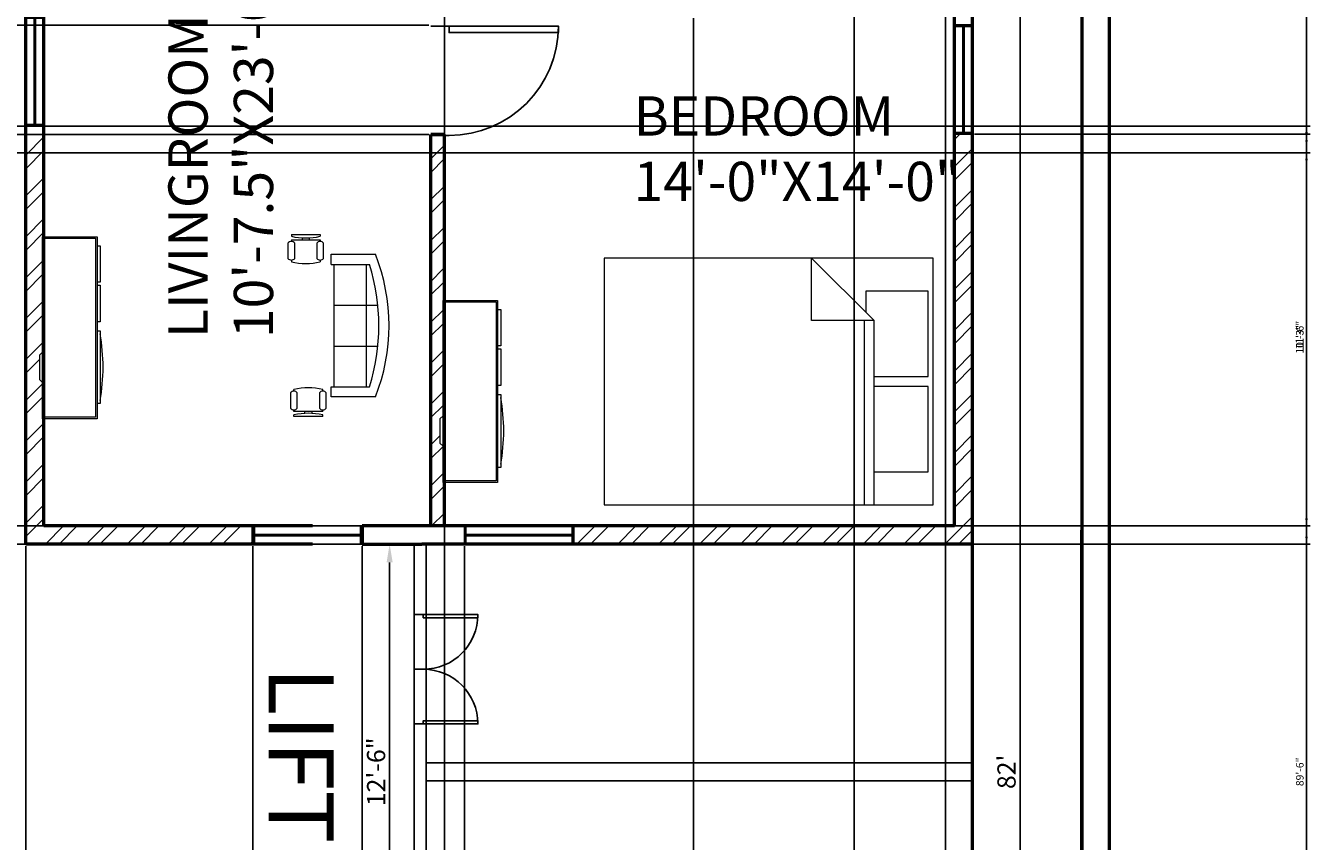
# Model space of a CAD drawing. Units: inches. Extents: x -12550 to 6516, y 1273 to 18700.
# Tile 6 of 19: x 2426 to 2849, y 1958 to 2227. Entities that reach past the tile are written whole.
import ezdxf

# ---------------------------------------------------------------- set-up
doc = ezdxf.new("R2010")
doc.units = ezdxf.units.IN
for name, color, linetype, lineweight in [('A-ANNO-DIMS', 2, 'Continuous', 18), ('A-AREA-IDEN', 1, 'Continuous', 18), ('A-DOOR', 5, 'Continuous', 25), ('A-EQPM', 4, 'Continuous', 25), ('A-FURN', 8, 'Continuous', 18), ('A-GLAZ', 3, 'Continuous', 25), ('A-WALL', 7, 'Continuous', 50), ('A-WALL-PATT', 8, 'Continuous', 13)]:
    doc.layers.add(name, color=color, linetype=linetype, lineweight=lineweight)
doc.styles.get("Standard").update_dxf_attribs({"font": 'arial.ttf'})
doc.dimstyles.new('ISO-25', dxfattribs={"dimtxt": 2.5, "dimasz": 2.5, "dimexe": 1.25, "dimexo": 0.625, "dimtad": 1, "dimlunit": 4, "dimtxsty": 'Standard', "dimcen": 2.5, "dimadec": 0, "dimazin": 0, "dimtfac": 1, "dimtmove": 0, "dimatfit": 3, "dimfxl": 1, "dimarcsym": 0})
pattern_1 = [(45, (-2e-13, 567), (-6.735192, 6.735192), []), (45, (4.49, 567), (-6.735192, 6.735192), [])]

# ---------------------------------------------------------------- blocks, each defined once
blk = doc.blocks.new('*U2')
for p, q in [((0, 0), (0, -5)), ((30, 0), (30, -5))]:
    blk.add_line(p, q)
blk.add_lwpolyline([(0, 0), (0, 30), (1.75, 30), (1.75, 0)], close=True)
blk.add_arc((0, 0), 30, 0, 90)
blk = doc.blocks.new('Bed - Queen')
for p, q in [((0, -80.00003), (0, 0)), ((0, 0), (59.99999, 0)), ((59.99999, 0), (59.99999, -80.00003)), ((7.99999, -1.2), (28.79998, -1.2)), ((7.99999, -14.4), (7.99999, -1.2)), ((28.79998, -1.2), (28.79998, -14.4)), ((31.19999, -1.2), (51.99999, -1.2)), ((31.19999, -14.4), (31.19999, -1.2)), ((51.99999, -1.2), (51.99999, -16.4)), ((0, -14.4), (44.8, -14.4)), ((59.99999, -29.6), (44.8, -14.4)), ((44.8, -14.4), (44.8, -29.6)), ((44.8, -16.8), (0, -16.8)), ((51.99999, -16.4), (46.79936, -16.4)), ((44.8, -29.6), (59.99999, -29.6)), ((59.99999, -80.00003), (0, -80.00003))]:
    blk.add_line(p, q)
blk = doc.blocks.new('Entertainment Center')
for p, q in [((-4, 0), (-5, -1)), ((4, 0), (-4, 0)), ((5, -1), (4, 0)), ((-17, -19), (-17, -1)), ((-17, -1), (43, -1)), ((-16.5, -18.5), (-16.5, -1.5)), ((-16.5, -1.5), (42.5, -1.5)), ((42.5, -1.5), (42.5, -18.5)), ((43, -1), (43, -19)), ((43, -19), (-17, -19)), ((42.5, -18.5), (-16.5, -18.5)), ((-12, -20), (-12, -19)), ((12, -20), (-12, -20)), ((12, -19), (12, -20)), ((15, -20), (15, -19)), ((27, -20), (15, -20)), ((27, -19), (27, -20)), ((28, -20), (28, -19)), ((40, -20), (28, -20)), ((40, -19), (40, -20))]:
    blk.add_line(p, q)
blk.add_arc((0, 40), 61, 259.6111, 280.3889)
blk = doc.blocks.new('Sofa - Roundback 7 ft.')
for p, q in [((-12.00002, -32.4421), (-12.00003, -6.5971)), ((11.99997, -32.4421), (11.99998, -6.5971)), ((-36.000027, -34), (-36.000027, -11.4696)), ((-35.999844, -13.3819), (35.9998, -13.3819)), ((35.99998, -34), (35.99998, -11.4696)), ((-36.000027, -32.4421), (35.99998, -32.4421))]:
    blk.add_line(p, q)
for points in [[(-36.000027, -34), (-42.000027, -34), (-42.000027, -8)], [(41.99998, -8), (41.99998, -34), (35.99998, -34)]]:
    blk.add_lwpolyline(points)
for centre, radius, start, end in [((0, -114.25), 114.25, 68.43141, 111.5686), ((-0.00001, -127.1968), 121.1968, 72.72033, 107.2797)]:
    blk.add_arc(centre, radius, start, end)
blk = doc.blocks.new('Chair - Desk')
for p, q in [((-8.5, 0), (-8.5, -1)), ((-8.5, 0), (8.5, 0)), ((8.5, 0), (8.5, -1)), ((-10.5, -5), (-10.5, -14)), ((-8.5, -3), (-8.5, -4)), ((-8.5, -3), (8.5, -3)), ((-6.5, -14), (-6.5, -5)), ((-2, -3), (-2, -1.9355)), ((2, -1.9576), (2, -3)), ((6.5, -5), (6.5, -14)), ((8.5, -3), (8.5, -4)), ((10.5, -14), (10.5, -5)), ((-8.5, -15), (-8.5, -16)), ((8.5, -15), (8.5, -16))]:
    blk.add_line(p, q)
for centre, radius, start, end in [((-8.5, -6.5), 2.5, 36.8699, 143.1301), ((0, 34.625), 36.625, 256.5803, 283.4197), ((8.5, -6.5), 2.5, 36.8699, 143.1301), ((-8.5, -12.5), 2.5, 216.8699, 323.1301), ((8.5, -12.5), 2.5, 216.8699, 323.1301), ((0, 19.625), 36.625, 256.5803, 283.4197)]:
    blk.add_arc(centre, radius, start, end)
blk = doc.blocks.new('*D14')
at = {"layer": 'A-ANNO-DIMS', "color": 0, "lineweight": -2, "transparency": 16777216}
for p, q in [((2553.06, 2056.25), (2544.35, 2056.25)), ((2545.6, 2050.25), (2545.6, 1912.25)), ((2553.06, 1906.25), (2544.35, 1906.25))]:
    blk.add_line(p, q, dxfattribs=at)
at = {"layer": 'A-ANNO-DIMS', "color": 0, "transparency": 16777216}
for points in [[(2544.6, 2050.25), (2546.6, 2050.25), (2545.6, 2056.25)], [(2544.6, 1912.25), (2546.6, 1912.25), (2545.6, 1906.25)]]:
    blk.add_solid(points, dxfattribs=at)
at = {"layer": 'Defpoints', "color": 0, "transparency": 16777216}
for p in [(2553.69, 2056.25), (2545.6, 1906.25), (2553.69, 1906.25)]:
    blk.add_point(p, dxfattribs=at)
at = {"layer": 'A-ANNO-DIMS', "color": 0, "transparency": 16777216, "insert": (2541.91, 1981.25), "char_height": 6, "attachment_point": 5, "rotation": 90}
blk.add_mtext('12\'-6"', dxfattribs=at)
blk = doc.blocks.new('*D16')
at = {"layer": 'A-ANNO-DIMS', "color": 0, "lineweight": -2, "transparency": 16777216}
for p, q in [((2738.31, 2473.25), (2754.56, 2473.25)), ((2753.31, 2467.25), (2753.31, 1495.25)), ((2738.31, 1489.25), (2754.56, 1489.25))]:
    blk.add_line(p, q, dxfattribs=at)
at = {"layer": 'A-ANNO-DIMS', "color": 0, "transparency": 16777216}
for points in [[(2752.31, 2467.25), (2754.31, 2467.25), (2753.31, 2473.25)], [(2752.31, 1495.25), (2754.31, 1495.25), (2753.31, 1489.25)]]:
    blk.add_solid(points, dxfattribs=at)
at = {"layer": 'Defpoints', "color": 0, "transparency": 16777216}
for p in [(2737.69, 2473.25), (2737.69, 1489.25), (2753.31, 1489.25)]:
    blk.add_point(p, dxfattribs=at)
at = {"layer": 'A-ANNO-DIMS', "color": 0, "transparency": 16777216, "insert": (2749.62, 1981.25), "char_height": 6, "attachment_point": 5, "rotation": 90}
blk.add_mtext("82'", dxfattribs=at)
blk = doc.blocks.new('WIN-3FT')
for p, q in [((0, 0), (0, 6)), ((0, 6), (36.02, 6)), ((0.5, 0), (0.5, 6)), ((35.52, 6), (35.52, 0)), ((36.02, 6), (36.02, 0)), ((36.02, 0), (0, 0)), ((35.52, 3.2), (0.5, 3.2)), ((35.52, 2.8), (0.5, 2.8))]:
    blk.add_line(p, q)
blk = doc.blocks.new('*D95')
at = {"layer": 'A-ANNO-DIMS', "color": 0, "lineweight": -2, "transparency": 16777216}
for p, q in [((2783.31, 2518.25), (2848.94, 2518.25)), ((2847.69, 1446.75), (2847.69, 2515.75)), ((2783.31, 1444.25), (2848.94, 1444.25))]:
    blk.add_line(p, q, dxfattribs=at)
at = {"layer": 'A-ANNO-DIMS', "color": 0, "transparency": 16777216}
for points in [[(2847.27, 2515.75), (2848.11, 2515.75), (2847.69, 2518.25)], [(2847.27, 1446.75), (2848.11, 1446.75), (2847.69, 1444.25)]]:
    blk.add_solid(points, dxfattribs=at)
at = {"layer": 'Defpoints', "color": 0, "transparency": 16777216}
for p in [(2782.69, 2518.25), (2847.69, 2518.25), (2782.69, 1444.25)]:
    blk.add_point(p, dxfattribs=at)
at = {"layer": 'A-ANNO-DIMS', "color": 0, "transparency": 16777216, "insert": (2845.79, 1981.25), "char_height": 2.5, "attachment_point": 5, "rotation": 90}
blk.add_mtext('89\'-6"', dxfattribs=at)
blk = doc.blocks.new('*D138')
at = {"layer": 'A-ANNO-DIMS', "color": 0, "lineweight": -2, "transparency": 16777216}
for p, q in [((2196.81, 2185.25), (2848.94, 2185.25)), ((2847.69, 2064.75), (2847.69, 2182.75)), ((2196.81, 2062.25), (2848.94, 2062.25))]:
    blk.add_line(p, q, dxfattribs=at)
at = {"layer": 'A-ANNO-DIMS', "color": 0, "transparency": 16777216}
for points in [[(2847.27, 2182.75), (2848.11, 2182.75), (2847.69, 2185.25)], [(2847.27, 2064.75), (2848.11, 2064.75), (2847.69, 2062.25)]]:
    blk.add_solid(points, dxfattribs=at)
at = {"layer": 'Defpoints', "color": 0, "transparency": 16777216}
for p in [(2196.19, 2185.25), (2847.69, 2185.25), (2196.19, 2062.25)]:
    blk.add_point(p, dxfattribs=at)
at = {"layer": 'A-ANNO-DIMS', "color": 0, "transparency": 16777216, "insert": (2845.79, 2123.75), "char_height": 2.5, "attachment_point": 5, "rotation": 90}
blk.add_mtext('10\'-3"', dxfattribs=at)
blk = doc.blocks.new('*D145')
at = {"layer": 'A-ANNO-DIMS', "color": 0, "lineweight": -2, "transparency": 16777216}
for p, q in [((2330.31, 2194.03), (2848.94, 2194.03)), ((2847.69, 2058.75), (2847.69, 2191.53)), ((2330.31, 2056.25), (2848.94, 2056.25))]:
    blk.add_line(p, q, dxfattribs=at)
at = {"layer": 'A-ANNO-DIMS', "color": 0, "transparency": 16777216}
for points in [[(2847.27, 2191.53), (2848.11, 2191.53), (2847.69, 2194.03)], [(2847.27, 2058.75), (2848.11, 2058.75), (2847.69, 2056.25)]]:
    blk.add_solid(points, dxfattribs=at)
at = {"layer": 'Defpoints', "color": 0, "transparency": 16777216}
for p in [(2329.69, 2194.03), (2847.69, 2194.03), (2329.69, 2056.25)]:
    blk.add_point(p, dxfattribs=at)
at = {"layer": 'A-ANNO-DIMS', "color": 0, "transparency": 16777216, "insert": (2845.79, 2125.14), "char_height": 2.5, "attachment_point": 5, "rotation": 90}
blk.add_mtext('11\'-6"', dxfattribs=at)
blk = doc.blocks.new('*D152')
at = {"layer": 'A-ANNO-DIMS', "color": 0, "lineweight": -2, "transparency": 16777216}
for p, q in [((2425.69, 2055.62), (2425.69, 1378)), ((2500.53, 2055.62), (2500.53, 1378)), ((2428.19, 1379.25), (2498.03, 1379.25))]:
    blk.add_line(p, q, dxfattribs=at)
at = {"layer": 'A-ANNO-DIMS', "color": 0, "transparency": 16777216}
for points in [[(2428.19, 1379.66), (2428.19, 1378.83), (2425.69, 1379.25)], [(2498.03, 1379.66), (2498.03, 1378.83), (2500.53, 1379.25)]]:
    blk.add_solid(points, dxfattribs=at)
at = {"layer": 'Defpoints', "color": 0, "transparency": 16777216}
for p in [(2425.69, 2056.25), (2500.53, 2056.25), (2500.53, 1379.25)]:
    blk.add_point(p, dxfattribs=at)
at = {"layer": 'A-ANNO-DIMS', "color": 0, "transparency": 16777216, "insert": (2463.11, 1381.15), "char_height": 2.5, "attachment_point": 5}
blk.add_mtext('6\'-3"', dxfattribs=at)
blk = doc.blocks.new('*D153')
at = {"layer": 'A-ANNO-DIMS', "color": 0, "lineweight": -2, "transparency": 16777216}
for p, q in [((2536.54, 2055.62), (2536.54, 1378)), ((2570.26, 2055.62), (2570.26, 1378)), ((2539.04, 1379.25), (2567.76, 1379.25))]:
    blk.add_line(p, q, dxfattribs=at)
at = {"layer": 'A-ANNO-DIMS', "color": 0, "transparency": 16777216}
for points in [[(2539.04, 1379.66), (2539.04, 1378.83), (2536.54, 1379.25)], [(2567.76, 1379.66), (2567.76, 1378.83), (2570.26, 1379.25)]]:
    blk.add_solid(points, dxfattribs=at)
at = {"layer": 'Defpoints', "color": 0, "transparency": 16777216}
for p in [(2536.54, 2056.25), (2570.26, 2056.25), (2570.26, 1379.25)]:
    blk.add_point(p, dxfattribs=at)
at = {"layer": 'A-ANNO-DIMS', "color": 0, "transparency": 16777216, "insert": (2553.4, 1381.16), "char_height": 2.5, "attachment_point": 5}
blk.add_mtext('2\'-9 1/2"', dxfattribs=at)
blk = doc.blocks.new('*D154')
at = {"layer": 'A-ANNO-DIMS', "color": 0, "lineweight": -2, "transparency": 16777216}
for p, q in [((2738.31, 2191.35), (2848.94, 2191.35)), ((2847.69, 2058.75), (2847.69, 2188.85)), ((2738.31, 2056.25), (2848.94, 2056.25))]:
    blk.add_line(p, q, dxfattribs=at)
at = {"layer": 'A-ANNO-DIMS', "color": 0, "transparency": 16777216}
for points in [[(2847.27, 2188.85), (2848.11, 2188.85), (2847.69, 2191.35)], [(2847.27, 2058.75), (2848.11, 2058.75), (2847.69, 2056.25)]]:
    blk.add_solid(points, dxfattribs=at)
at = {"layer": 'Defpoints', "color": 0, "transparency": 16777216}
for p in [(2737.69, 2191.35), (2847.69, 2191.35), (2737.69, 2056.25)]:
    blk.add_point(p, dxfattribs=at)
at = {"layer": 'A-ANNO-DIMS', "color": 0, "transparency": 16777216, "insert": (2845.79, 2123.8), "char_height": 2.5, "attachment_point": 5, "rotation": 90}
blk.add_mtext('11\'-3"', dxfattribs=at)
blk = doc.blocks.new('*D157')
at = {"layer": 'A-ANNO-DIMS', "color": 0, "lineweight": -2, "transparency": 16777216}
for p, q in [((2558.56, 2191.25), (1906.44, 2191.25)), ((1907.69, 2064.75), (1907.69, 2188.75)), ((2558.56, 2062.25), (1906.44, 2062.25))]:
    blk.add_line(p, q, dxfattribs=at)
at = {"layer": 'A-ANNO-DIMS', "color": 0, "transparency": 16777216}
for points in [[(1907.27, 2188.75), (1908.11, 2188.75), (1907.69, 2191.25)], [(1907.27, 2064.75), (1908.11, 2064.75), (1907.69, 2062.25)]]:
    blk.add_solid(points, dxfattribs=at)
at = {"layer": 'Defpoints', "color": 0, "transparency": 16777216}
for p in [(1907.69, 2191.25), (2559.19, 2191.25), (2559.19, 2062.25)]:
    blk.add_point(p, dxfattribs=at)
at = {"layer": 'A-ANNO-DIMS', "color": 0, "transparency": 16777216, "insert": (1905.79, 2126.75), "char_height": 2.5, "attachment_point": 5, "rotation": 90}
blk.add_mtext('10\'-9"', dxfattribs=at)
blk = doc.blocks.new('*D158')
at = {"layer": 'A-ANNO-DIMS', "color": 0, "lineweight": -2, "transparency": 16777216}
for p, q in [((2558.56, 2227.25), (1906.44, 2227.25)), ((1907.69, 2193.75), (1907.69, 2224.75)), ((2558.56, 2191.25), (1906.44, 2191.25))]:
    blk.add_line(p, q, dxfattribs=at)
at = {"layer": 'A-ANNO-DIMS', "color": 0, "transparency": 16777216}
for points in [[(1907.27, 2224.75), (1908.11, 2224.75), (1907.69, 2227.25)], [(1907.27, 2193.75), (1908.11, 2193.75), (1907.69, 2191.25)]]:
    blk.add_solid(points, dxfattribs=at)
at = {"layer": 'Defpoints', "color": 0, "transparency": 16777216}
for p in [(1907.69, 2227.25), (2559.19, 2227.25), (2559.19, 2191.25)]:
    blk.add_point(p, dxfattribs=at)
at = {"layer": 'A-ANNO-DIMS', "color": 0, "transparency": 16777216, "insert": (1905.79, 2209.25), "char_height": 2.5, "attachment_point": 5, "rotation": 90}
blk.add_mtext('3\'-0"', dxfattribs=at)
blk = doc.blocks.new('*D162')
at = {"layer": 'A-ANNO-DIMS', "color": 0, "lineweight": -2, "transparency": 16777216}
for p, q in [((2698.69, 2234.12), (2698.69, 1378)), ((2728.69, 2234.12), (2728.69, 1378)), ((2701.19, 1379.25), (2726.19, 1379.25))]:
    blk.add_line(p, q, dxfattribs=at)
at = {"layer": 'A-ANNO-DIMS', "color": 0, "transparency": 16777216}
for points in [[(2701.19, 1379.66), (2701.19, 1378.83), (2698.69, 1379.25)], [(2726.19, 1379.66), (2726.19, 1378.83), (2728.69, 1379.25)]]:
    blk.add_solid(points, dxfattribs=at)
at = {"layer": 'Defpoints', "color": 0, "transparency": 16777216}
for p in [(2698.69, 2234.75), (2728.69, 2234.75), (2728.69, 1379.25)]:
    blk.add_point(p, dxfattribs=at)
at = {"layer": 'A-ANNO-DIMS', "color": 0, "transparency": 16777216, "insert": (2713.69, 1381.15), "char_height": 2.5, "attachment_point": 5}
blk.add_mtext('2\'-6"', dxfattribs=at)
blk = doc.blocks.new('*D163')
at = {"layer": 'A-ANNO-DIMS', "color": 0, "lineweight": -2, "transparency": 16777216}
for p, q in [((2563.69, 2234.12), (2563.69, 1378)), ((2645.69, 2229.62), (2645.69, 1378)), ((2566.19, 1379.25), (2643.19, 1379.25))]:
    blk.add_line(p, q, dxfattribs=at)
at = {"layer": 'A-ANNO-DIMS', "color": 0, "transparency": 16777216}
for points in [[(2566.19, 1379.66), (2566.19, 1378.83), (2563.69, 1379.25)], [(2643.19, 1379.66), (2643.19, 1378.83), (2645.69, 1379.25)]]:
    blk.add_solid(points, dxfattribs=at)
at = {"layer": 'Defpoints', "color": 0, "transparency": 16777216}
for p in [(2563.69, 2234.75), (2645.69, 2230.25), (2645.69, 1379.25)]:
    blk.add_point(p, dxfattribs=at)
at = {"layer": 'A-ANNO-DIMS', "color": 0, "transparency": 16777216, "insert": (2604.69, 1381.15), "char_height": 2.5, "attachment_point": 5}
blk.add_mtext('6\'-10"', dxfattribs=at)

msp = doc.modelspace()

# ---------------------------------------------------------------- hatches: boundary and pattern name
at = {"layer": 'A-WALL-PATT'}
h = msp.add_hatch(dxfattribs=at)
h.set_pattern_fill('ANSI32', color=256)
h.set_pattern_definition(pattern_1)
h.paths.add_polyline_path([(2500.528, 2056.247), (2500.528, 2062.247), (2431.689, 2062.247), (2431.689, 2097.559), (2431.189, 2097.559), (2431.189, 2109.559), (2430.189, 2110.559), (2430.189, 2118.559), (2431.189, 2119.559), (2431.189, 2157.559), (2431.689, 2157.559), (2431.689, 2194.032), (2425.689, 2194.032), (2425.689, 2056.247)])
h = msp.add_hatch(dxfattribs=at)
h.set_pattern_fill('ANSI32', color=256)
h.set_pattern_definition(pattern_1)
h.paths.add_polyline_path([(2559.189, 2190.947), (2559.189, 2062.247), (2563.689, 2062.247), (2563.689, 2076.575), (2563.189, 2076.575), (2563.189, 2088.575), (2562.189, 2089.575), (2562.189, 2097.575), (2563.189, 2098.575), (2563.189, 2136.575), (2563.686, 2190.947)])
h = msp.add_hatch(dxfattribs=at)
h.set_pattern_fill('ANSI32', color=256)
h.set_pattern_definition(pattern_1)
h.paths.add_polyline_path([(2737.689, 2191.352), (2731.689, 2191.352), (2731.689, 2062.247), (2606.275, 2062.247), (2606.275, 2056.247), (2737.689, 2056.247)])

# ---------------------------------------------------------------- linework, layer by layer
at = {"layer": 'A-EQPM'}
for p, q in [((2553.689, 1906.247), (2553.689, 2056.247)), ((2737.689, 2056.247), (2553.689, 2056.247)), ((2557.689, 1906.247), (2557.689, 2056.247)), ((2737.689, 2056.247), (2737.689, 1906.247)), ((2737.689, 1984.247), (2557.689, 1984.247)), ((2737.689, 1978.247), (2557.689, 1978.247))]:
    msp.add_line(p, q, dxfattribs=at)
at = {"layer": 'A-WALL'}
for p, q in [((2782.689, 2518.247), (2782.689, 1444.247)), ((2773.689, 2509.247), (2773.689, 1453.247)), ((2737.689, 2060.923), (2737.689, 2473.247)), ((2425.689, 2056.247), (2425.689, 2234.747)), ((2431.689, 2062.247), (2431.689, 2234.747)), ((2731.689, 2062.247), (2731.689, 2230.247)), ((2559.189, 2062.247), (2559.189, 2191.247)), ((2563.689, 2191.247), (2559.189, 2191.247)), ((2563.689, 2062.247), (2563.689, 2191.247)), ((2520.189, 2062.247), (2431.689, 2062.247)), ((2500.528, 2062.247), (2500.528, 2056.247)), ((2536.545, 2062.247), (2536.545, 2056.247)), ((2556.189, 2062.247), (2536.545, 2062.247)), ((2731.689, 2062.247), (2556.189, 2062.247)), ((2559.189, 2062.247), (2556.189, 2062.247)), ((2737.689, 1489.247), (2737.689, 2060.923)), ((2773.689, 1489.247), (2773.689, 2060.923)), ((2520.189, 2056.247), (2425.689, 2056.247)), ((2536.545, 2056.247), (2556.189, 2056.247)), ((2737.689, 2056.247), (2556.189, 2056.247))]:
    msp.add_line(p, q, dxfattribs=at)

# ---------------------------------------------------------------- block references
at = {"layer": 'A-DOOR', "xscale": 1.199999999999999, "yscale": 1.199999999999999, "zscale": 1.199999999999999, "rotation": 270}
msp.add_blockref('*U2', (2565.189, 2226.947), dxfattribs=at)
at = {"layer": 'A-EQPM', "yscale": 0.5999999999999954, "zscale": 0.5999999999999954, "rotation": 270}
for p, xscale in [((2556.689, 2033.042), 0.5999999999999954), ((2556.689, 1997.042), -0.5999999999999954)]:
    msp.add_blockref('*U2', p, dxfattribs=dict(at, xscale=xscale))
at = {"layer": 'A-FURN', "rotation": 89.99999999999999}
for p in [(2430.189, 2114.559), (2562.189, 2093.575)]:
    msp.add_blockref('Entertainment Center', p, dxfattribs=at)
at = {"layer": 'A-FURN', "xscale": 0.5595223685495907, "yscale": 0.5595223685495907, "zscale": 0.5595223685495907}
msp.add_blockref('Chair - Desk', (2517.969, 2158.265), dxfattribs=at)
at = {"layer": 'A-FURN'}
for name, p, xscale, yscale, zscale, rotation in [('Sofa - Roundback 7 ft.', (2545.408, 2128.265), 0.5595223685495907, 0.5595223685495907, 0.5595223685495907, 270), ('Bed - Queen', (2724.708, 2069.217), -1.354827908062564, 1.354827908062564, 1.354827908062564, 270), ('Chair - Desk', (2518.822, 2098.281), 0.5595223685495907, 0.5595223685495907, 0.5595223685495907, 180)]:
    msp.add_blockref(name, p, dxfattribs=dict(at, xscale=xscale, yscale=yscale, zscale=zscale, rotation=rotation))
at = {"layer": 'A-GLAZ'}
for p, rotation in [((2431.689, 2194.032), 90.00000000000047), ((2737.689, 2191.352), 90.00000000000047), ((2536.545, 2062.247), 180), ((2606.275, 2062.247), 180)]:
    msp.add_blockref('WIN-3FT', p, dxfattribs=dict(at, rotation=rotation))

# ---------------------------------------------------------------- texts
at = {"layer": 'A-AREA-IDEN', "insert": (2472.713, 2124.153), "char_height": 12.93169, "attachment_point": 1, "rotation": 90}
msp.add_mtext('LIVINGROOM\\P10\'-7.5"X23\'-0"', dxfattribs=at)
at = {"layer": 'A-AREA-IDEN', "insert": (2625.969, 2203.812), "char_height": 12.93169, "attachment_point": 1}
msp.add_mtext('BEDROOM\\P14\'-0"X14\'-0"', dxfattribs=at)
at = {"layer": 'A-AREA-IDEN', "insert": (2527.176, 2015.823), "char_height": 21.4543, "attachment_point": 1, "rotation": 270}
msp.add_mtext_dynamic_manual_height_columns('LIFT', width=3.27433, gutter_width=107.272, heights=[0], dxfattribs=at)

# ---------------------------------------------------------------- dimensions: what is measured, and where the dimension line sits
at = {"layer": 'A-ANNO-DIMS'}
for base, p1, p2, override, picture, middle in [((2847.689, 2518.247), (2782.689, 1444.247), (2782.689, 2518.247), {"dimdec": 1, "dimlfac": 1, "dimrnd": 0, "dimzin": 1, "dimdsep": 46, "dimlunit": 4, "dimfrac": 2}, '*D95', (2845.787, 1981.247)), ((2753.309, 1489.247), (2737.689, 2473.247), (2737.689, 1489.247), {"dimtxt": 6, "dimasz": 6, "dimclrd": 0, "dimclre": 0, "dimclrt": 0}, '*D16', (2749.62, 1981.247)), ((1907.689, 2227.247), (2559.189, 2191.247), (2559.189, 2227.247), {"dimdec": 1, "dimlfac": 1, "dimrnd": 0, "dimzin": 1, "dimdsep": 46, "dimlunit": 4, "dimfrac": 2}, '*D158', (1905.787, 2209.247)), ((2847.689, 2194.032), (2329.689, 2056.247), (2329.689, 2194.032), {"dimdec": 1, "dimlfac": 1, "dimrnd": 0, "dimzin": 1, "dimdsep": 46, "dimlunit": 4, "dimfrac": 2}, '*D145', (2845.787, 2125.14)), ((1907.689, 2191.247), (2559.189, 2062.247), (2559.189, 2191.247), {"dimdec": 1, "dimlfac": 1, "dimrnd": 0, "dimzin": 1, "dimdsep": 46, "dimlunit": 4, "dimfrac": 2}, '*D157', (1905.787, 2126.747)), ((2847.689, 2191.352), (2737.689, 2056.247), (2737.689, 2191.352), {"dimdec": 1, "dimlfac": 1, "dimrnd": 0, "dimzin": 1, "dimdsep": 46, "dimlunit": 4, "dimfrac": 2}, '*D154', (2845.787, 2123.8)), ((2847.689, 2185.247), (2196.189, 2062.247), (2196.189, 2185.247), {"dimdec": 1, "dimlfac": 1, "dimrnd": 0, "dimzin": 1, "dimdsep": 46, "dimlunit": 4, "dimfrac": 2}, '*D138', (2845.787, 2123.747)), ((2545.602, 1906.247), (2553.689, 2056.247), (2553.689, 1906.247), {"dimtxt": 6, "dimasz": 6, "dimclrd": 0, "dimclre": 0, "dimclrt": 0}, '*D14', (2541.914, 1981.247))]:
    dim = msp.add_linear_dim(base=base, p1=p1, p2=p2, angle=90, dimstyle='ISO-25', override=override, dxfattribs=at)
    dim.commit()
    dim.dimension.update_dxf_attribs({"geometry": picture, "text_midpoint": middle})
for base, p1, p2, picture, middle in [((2645.689, 1379.247), (2563.689, 2234.747), (2645.689, 2230.247), '*D163', (2604.689, 1381.149)), ((2728.689, 1379.247), (2698.689, 2234.747), (2728.689, 2234.747), '*D162', (2713.689, 1381.149)), ((2500.528, 1379.247), (2425.689, 2056.247), (2500.528, 2056.247), '*D152', (2463.108, 1381.15)), ((2570.258, 1379.247), (2536.545, 2056.247), (2570.258, 2056.247), '*D153', (2553.401, 1381.165))]:
    dim = msp.add_linear_dim(base=base, p1=p1, p2=p2, dimstyle='ISO-25', override={"dimdec": 1, "dimlfac": 1, "dimrnd": 0, "dimzin": 1, "dimdsep": 46, "dimlunit": 4, "dimfrac": 2}, dxfattribs=at)
    dim.commit()
    dim.dimension.update_dxf_attribs({"geometry": picture, "text_midpoint": middle})

doc.saveas('drawing.dxf')
